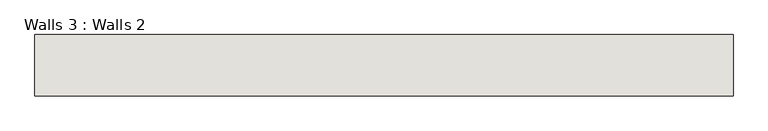
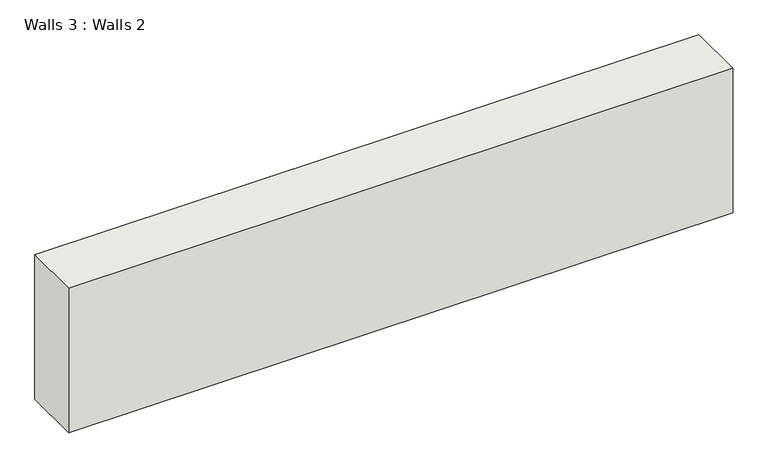
"""IFC4 building model written with IfcOpenShell, lengths in millimetres: wall geometry, Walls 3 : Walls 2."""

from ifc_helpers import new_model, si_unit, frame, origin, place, context, project, spatial, polyline, outline, extrude, source, transform, mapped, element, save


def walls_3_walls_2_f167fe74(model_context):
    return source(origin(), model_context, "Body", "SweptSolid", [
        extrude(outline(polyline([(-1482.6998814, 272.7610824), (-5851.4998814, 272.7610824), (-5851.4998814, 656.4749382), (-1482.6998814, 656.4749382), (-1482.6998814, 272.7610824)])), frame((0.0, 0.0, 14257.0380846), z_axis=(0.0, 0.0, 1.0), x_axis=(1.0, 0.0, 0.0)), (0.0, 0.0, 1.0), 1003.8673686),
    ])


if __name__ == "__main__":
    model = new_model("IFC4")
    model_context = context("Model", 3, world=origin())
    ifc_project = project(units=[si_unit("LENGTHUNIT", "METRE", prefix="MILLI")], contexts=[model_context])
    site = spatial("IfcSite", under=ifc_project)
    building = spatial("IfcBuilding", under=site)
    placement = place(None, origin())
    walls_3_walls_2_shape = walls_3_walls_2_f167fe74(model_context)
    element("IfcWall", 1, ObjectType="Walls 3 : Walls 2", at=placement, inside=building, context=model_context, shape_type="MappedRepresentation", body=[
        mapped(walls_3_walls_2_shape, transform((0.0, 0.0, 0.0), x_axis=(1.0, 0.0, 0.0), y_axis=(0.0, 1.0, 0.0), z_axis=(0.0, 0.0, 1.0))),
    ])
    save(model, "model.ifc")

# Revit data of these elements
# Element 1 (IfcWall, "Walls 3 : Walls 2")
#   Materials on its faces: "Default Wall"
# Materials
#   "Default Wall": colour RGB 128 128 128, transparency 0
